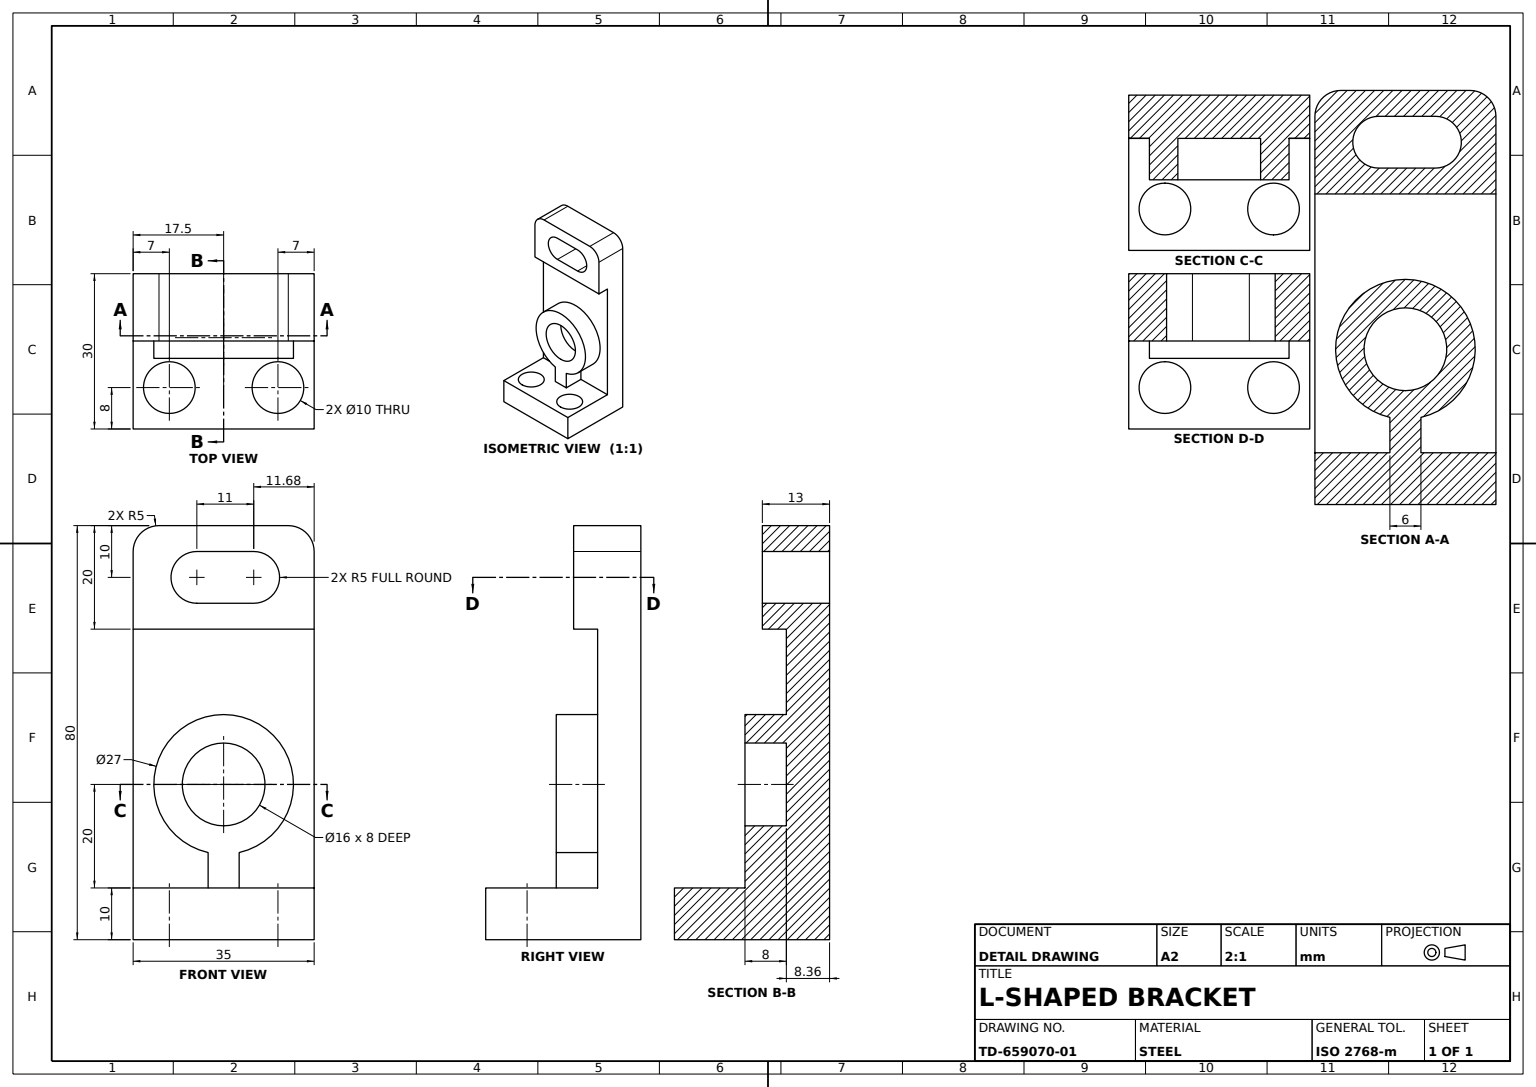
SolidWorks part; units mm, degrees
material "Plain Carbon Steel"
ref_plane "Front Plane" through (0, 0, 0) normal (0, 0, 1) x (1, 0, 0)
ref_plane "Top Plane" through (0, 0, 0) normal (0, 1, 0) x (1, 0, 0)
ref_plane "Right Plane" through (0, 0, 0) normal (1, 0, 0) x (0, 0, -1)
sketch "Bracket Profile Sketch" plane through (0, 0, 0) normal (1, 0, 0) x (0, 0, -1)
  line L1 (-17.5, 40) -> (17.5, 40)
  line L2 (-17.5, 40) -> (-17.5, -40)
  line L3 (-17.5, -40) -> (17.5, -40)
  line L4 (17.5, 40) -> (17.5, -40)
  line L5 (-17.5, 40) -> (17.5, -40) construction
  line L6 (-17.5, -40) -> (17.5, 40) construction
  point P0 (0, 0)
  dimension "D1" = 80
  dimension "D2" = 35
extrude "Bracket Body" add sketch "Bracket Profile Sketch" along normal blind 30
sketch "Side Relief Sketch" plane through (0, 0, 17.5) normal (0, 0, 1) x (1, 0, 0)
  line L0 (13, 40) -> (13, 20)
  line L1 (30, 40) -> (0, 40) construction
  line L2 (13, 20) -> (8.3587, 20)
  line L3 (8.3587, 20) -> (8.3587, -30)
  line L4 (8.3587, -30) -> (30, -30)
  line L5 (30, 40) -> (30, -40) construction
  line L6 (30, -30) -> (30, 40)
  line L7 (30, 40) -> (13, 40)
  line L8 (0, 40) -> (0, -40) construction
  line L9 (30, -40) -> (0, -40) construction
  dimension "D1" = 13
  dimension "D2" = 20
  dimension "D3" = 8.3587
  dimension "D4" = 10
extrude "Side Relief Cut" cut sketch "Side Relief Sketch" against normal through all
sketch "Ring Boss Sketch" plane through (8.3587, 0, 0) normal (1, 0, 0) x (0, 0, -1)
  line L0 (17.5, -30) -> (-17.5, -30) construction
  line L1 (-17.5, 20) -> (-17.5, -30) construction
  line L2 (-3, -30) -> (3, -30)
  line L3 (-3, -30) -> (-3, -23.1624)
  line L5 (3, -30) -> (3, -23.1624)
  arc A0 (3, -23.1624) -> (-3, -23.1624) centre (0, -10) ccw
  dimension "D1" = 27
  dimension "D2" = 20
  dimension "D3" = 6
  dimension "D4" = 17.5
extrude "Ring Boss" add sketch "Ring Boss Sketch" along normal blind 8 contours A0 L3 L2 L5
sketch "Boss Bore Sketch" plane through (16.3587, 0, 0) normal (1, 0, 0) x (0, 0, -1)
  circle A0 centre (0, -10) radius 8
  dimension "D1" = 16
extrude "Boss Bore Ø16" cut sketch "Boss Bore Sketch" against normal blind 8
sketch "Base Holes Sketch" plane through (0, -30, 0) normal (0, 1, 0) x (1, 0, 0)
  line L0 (30, 17.5) -> (30, -17.5) construction
  line L1 (8.3587, 17.5) -> (30, 17.5) construction
  line L2 (36.1187, 0) -> (-2.8991, 0) construction
  circle A0 centre (22, 10.5) radius 5
  circle A1 centre (22, -10.5) radius 5
  dimension "D3" = 10
  dimension "D1" = 8
  dimension "D2" = 7
extrude "Base Holes" cut sketch "Base Holes Sketch" against normal through all
fillet "Edge Fillet R5" radius 5 2 edges at (6.5, 40, -17.5) (6.5, 40, 17.5)
sketch "Top Slot Sketch" plane through (13, 0, 0) normal (1, 0, 0) x (0, 0, -1)
  line L0 (-5.181, 30) -> (5.819, 30) construction
  line L1 (-5.181, 35) -> (5.819, 35)
  line L2 (-5.181, 25) -> (5.819, 25)
  line L3 (0, 45.5919) -> (0, 14.5633) construction
  line L4 (-27.1183, 30) -> (25.9299, 30) construction
  line L5 (12.5, 40) -> (-12.5, 40) construction
  arc A0 (-5.181, 35) -> (-5.181, 25) centre (-5.181, 30) ccw
  arc A1 (5.819, 25) -> (5.819, 35) centre (5.819, 30) ccw
  point P2 (0.319, 30)
  dimension "D1" = 11
  dimension "D2" = 10
  dimension "D3" = 10
  dimension "D4" = 11.681
extrude "Top Slot Cut" cut sketch "Top Slot Sketch" against normal through all
